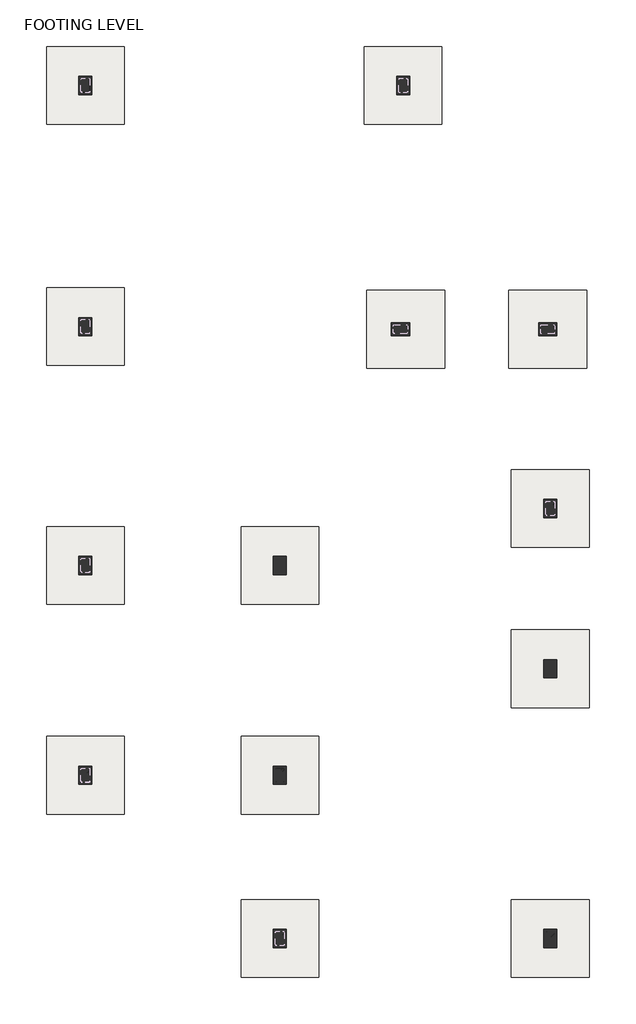
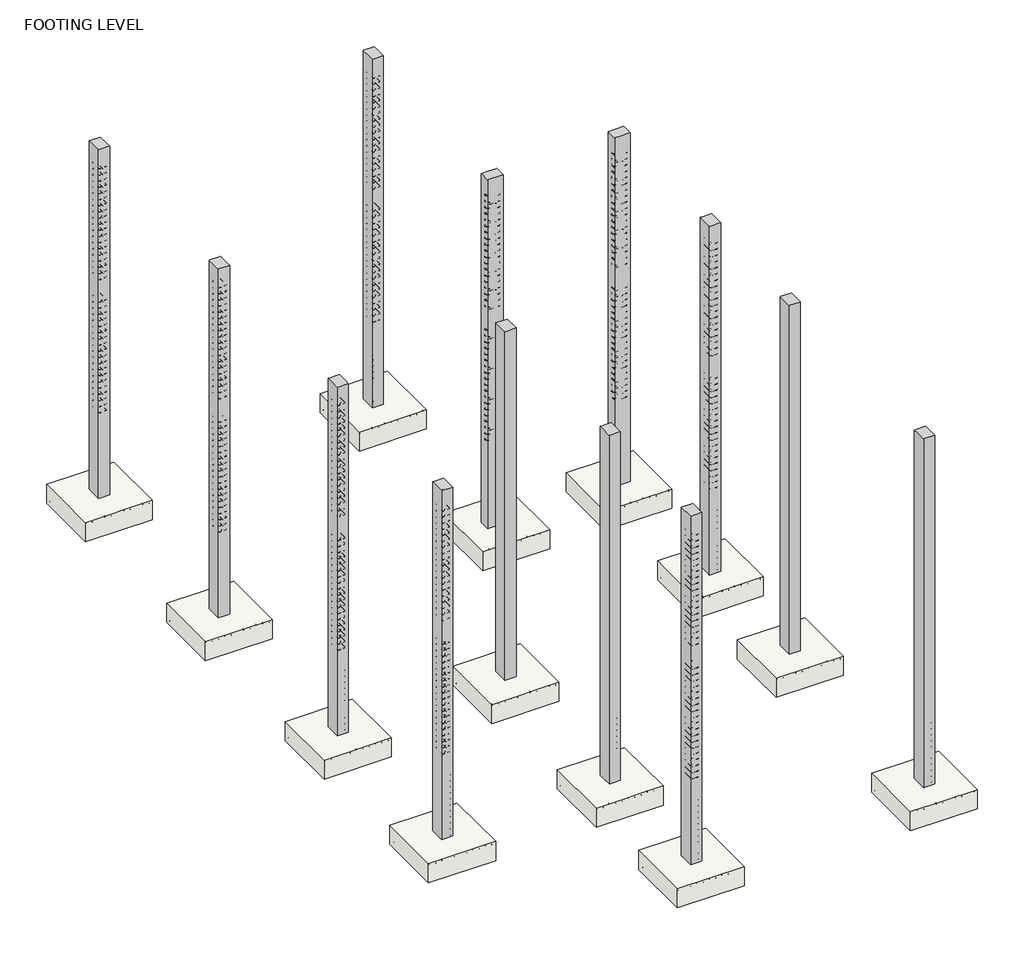
# One storey, part 1 of 9: 13 columns, 13 slabs.
"""IFC4 building model written with IfcOpenShell, lengths in millimetres."""

from ifc_helpers import new_model, si_unit, origin, place, context, project, spatial, faceted_brep, transform, mapped, element, save
from components import footing_rectangular_5_x_5_df1ede25

model = new_model("IFC4")

# Units and contexts
model_context = context("Model", 3, world=origin())
ifc_project = project(units=[si_unit("LENGTHUNIT", "METRE", prefix="MILLI")], contexts=[model_context])

# Site, building, storey
site = spatial("IfcSite", under=ifc_project)
building = spatial("IfcBuilding", under=site)
storey = spatial("IfcBuildingStorey", under=building, Name="FOOTING LEVEL", Elevation=-1981.2)

# Columns
placement = place(None, origin())
element("IfcColumn", 1, ObjectType="Concrete-Rectangular-Column : 10\" x 14\"", at=placement, inside=storey, context=model_context, shape_type="Brep", body=[
    faceted_brep([(-12235.0833659, -383.2216598, -1981.2), (-12235.0833659, -738.8216598, -1981.2), (-12489.0833659, -738.8216598, -1981.2), (-12489.0833659, -383.2216598, -1981.2), (-12235.0833659, -383.2216598, 6400.8), (-12235.0833659, -497.5216598, 6400.8), (-12235.0833659, -726.1216598, 6400.8), (-12235.0833659, -738.8216598, 6400.8), (-12489.0833659, -738.8216598, 6400.8), (-12489.0833659, -383.2216598, 6400.8), (-12476.3833659, -383.2216598, 6400.8), (-12247.7833659, -383.2216598, 6400.8)], [[[0, 1, 2, 3]], [[4, 5, 6, 7, 1, 0]], [[7, 8, 2, 1]], [[8, 9, 3, 2]], [[9, 10, 11, 4, 0, 3]], [[4, 11, 10, 9, 8, 7, 6, 5]]]),
])
element("IfcColumn", 2, ObjectType="Concrete-Rectangular-Column : 10\" x 14\"", at=placement, inside=storey, context=model_context, shape_type="Brep", body=[
    faceted_brep([(-12235.0833659, 3725.2283402, -1981.2), (-12235.0833659, 3369.6283402, -1981.2), (-12489.0833659, 3369.6283402, -1981.2), (-12489.0833659, 3725.2283402, -1981.2), (-12235.0833659, 3725.2283402, 6400.8), (-12235.0833659, 3712.5283402, 6400.8), (-12235.0833659, 3483.9283402, 6400.8), (-12235.0833659, 3369.6283402, 6400.8), (-12247.7833659, 3369.6283402, 6400.8), (-12476.3833659, 3369.6283402, 6400.8), (-12489.0833659, 3369.6283402, 6400.8), (-12489.0833659, 3725.2283402, 6400.8), (-12476.3833659, 3725.2283402, 6400.8), (-12247.7833659, 3725.2283402, 6400.8)], [[[0, 1, 2, 3]], [[4, 5, 6, 7, 1, 0]], [[7, 8, 9, 10, 2, 1]], [[10, 11, 3, 2]], [[11, 12, 13, 4, 0, 3]], [[4, 13, 12, 11, 10, 9, 8, 7, 6, 5]]]),
])
element("IfcColumn", 3, ObjectType="Concrete-Rectangular-Column : 10\" x 14\"", at=placement, inside=storey, context=model_context, shape_type="Brep", body=[
    faceted_brep([(-8425.0833659, 3725.2283402, -1981.2), (-8425.0833659, 3369.6283402, -1981.2), (-8679.0833659, 3369.6283402, -1981.2), (-8679.0833659, 3725.2283402, -1981.2), (-8425.0833659, 3725.2283402, 6400.8), (-8425.0833659, 3369.6283402, 6400.8), (-8437.7833659, 3369.6283402, 6400.8), (-8666.3833659, 3369.6283402, 6400.8), (-8679.0833659, 3369.6283402, 6400.8), (-8679.0833659, 3483.9283402, 6400.8), (-8679.0833659, 3712.5283402, 6400.8), (-8679.0833659, 3725.2283402, 6400.8)], [[[0, 1, 2, 3]], [[4, 5, 1, 0]], [[5, 6, 7, 8, 2, 1]], [[8, 9, 10, 11, 3, 2]], [[11, 4, 0, 3]], [[4, 11, 10, 9, 8, 7, 6, 5]]]),
])
element("IfcColumn", 4, ObjectType="Concrete-Rectangular-Column : 10\" x 14\"", at=placement, inside=storey, context=model_context, shape_type="Brep", body=[
    faceted_brep([(-3129.3191189, 1700.3598175, -1981.2), (-3129.3191189, 1344.7598175, -1981.2), (-3383.3191189, 1344.7598175, -1981.2), (-3383.3191189, 1700.3598175, -1981.2), (-3129.3191189, 1700.3598175, 6400.8), (-3129.3191189, 1344.7598175, 6400.8), (-3142.0191189, 1344.7598175, 6400.8), (-3370.6191189, 1344.7598175, 6400.8), (-3383.3191189, 1344.7598175, 6400.8), (-3383.3191189, 1700.3598175, 6400.8), (-3370.6191189, 1700.3598175, 6400.8), (-3142.0191189, 1700.3598175, 6400.8)], [[[0, 1, 2, 3]], [[4, 5, 1, 0]], [[5, 6, 7, 8, 2, 1]], [[8, 9, 3, 2]], [[9, 10, 11, 4, 0, 3]], [[4, 11, 10, 9, 8, 7, 6, 5]]]),
])
element("IfcColumn", 5, ObjectType="Concrete-Rectangular-Column : 10\" x 14\"", at=placement, inside=storey, context=model_context, shape_type="Brep", body=[
    faceted_brep([(-3129.3191189, -3583.6216598, -1981.2), (-3129.3191189, -3939.2216598, -1981.2), (-3383.3191189, -3939.2216598, -1981.2), (-3383.3191189, -3583.6216598, -1981.2), (-3129.3191189, -3583.6216598, 6400.8), (-3129.3191189, -3939.2216598, 6400.8), (-3383.3191189, -3939.2216598, 6400.8), (-3383.3191189, -3926.5216598, 6400.8), (-3383.3191189, -3697.9216598, 6400.8), (-3383.3191189, -3583.6216598, 6400.8), (-3370.6191189, -3583.6216598, 6400.8), (-3142.0191189, -3583.6216598, 6400.8)], [[[0, 1, 2, 3]], [[4, 5, 1, 0]], [[5, 6, 2, 1]], [[6, 7, 8, 9, 3, 2]], [[9, 10, 11, 4, 0, 3]], [[4, 11, 10, 9, 8, 7, 6, 5]]]),
])
element("IfcColumn", 6, ObjectType="Concrete-Rectangular-Column : 10\" x 14\"", at=placement, inside=storey, context=model_context, shape_type="Brep", body=[
    faceted_brep([(-8425.0833659, -3583.6216598, -1981.2), (-8425.0833659, -3939.2216598, -1981.2), (-8679.0833659, -3939.2216598, -1981.2), (-8679.0833659, -3583.6216598, -1981.2), (-8425.0833659, -3583.6216598, 6400.8), (-8425.0833659, -3697.9216598, 6400.8), (-8425.0833659, -3926.5216598, 6400.8), (-8425.0833659, -3939.2216598, 6400.8), (-8679.0833659, -3939.2216598, 6400.8), (-8679.0833659, -3583.6216598, 6400.8), (-8666.3833659, -3583.6216598, 6400.8), (-8437.7833659, -3583.6216598, 6400.8)], [[[0, 1, 2, 3]], [[4, 5, 6, 7, 1, 0]], [[7, 8, 2, 1]], [[8, 9, 3, 2]], [[9, 10, 11, 4, 0, 3]], [[4, 11, 10, 9, 8, 7, 6, 5]]]),
])
element("IfcColumn", 7, ObjectType="Concrete-Rectangular-Column : 10\" x 14\"", at=placement, inside=storey, context=model_context, shape_type="Brep", body=[
    faceted_brep([(-3129.3191189, 4841.8494441, -1981.2), (-3129.3191189, 4486.2494441, -1981.2), (-3383.3191189, 4486.2494441, -1981.2), (-3383.3191189, 4841.8494441, -1981.2), (-3129.3191189, 4841.8494441, 6400.8), (-3129.3191189, 4486.2494441, 6400.8), (-3142.0191189, 4486.2494441, 6400.8), (-3370.6191189, 4486.2494441, 6400.8), (-3383.3191189, 4486.2494441, 6400.8), (-3383.3191189, 4841.8494441, 6400.8), (-3370.6191189, 4841.8494441, 6400.8), (-3142.0191189, 4841.8494441, 6400.8)], [[[0, 1, 2, 3]], [[4, 5, 1, 0]], [[5, 6, 7, 8, 2, 1]], [[8, 9, 3, 2]], [[9, 10, 11, 4, 0, 3]], [[4, 11, 10, 9, 8, 7, 6, 5]]]),
])
element("IfcColumn", 8, ObjectType="Concrete-Rectangular-Column : 10\" x 14\"", at=placement, inside=storey, context=model_context, shape_type="Brep", body=[
    faceted_brep([(-3484.7833659, 8303.5783402, -1981.2), (-3129.1833659, 8303.5783402, -1981.2), (-3129.1833659, 8049.5783402, -1981.2), (-3484.7833659, 8049.5783402, -1981.2), (-3484.7833659, 8303.5783402, 6400.8), (-3129.1833659, 8303.5783402, 6400.8), (-3129.1833659, 8049.5783402, 6400.8), (-3142.0191189, 8049.5783402, 6400.8), (-3370.6191189, 8049.5783402, 6400.8), (-3484.7833659, 8049.5783402, 6400.8), (-3484.7833659, 8062.2783402, 6400.8), (-3484.7833659, 8290.8783402, 6400.8)], [[[0, 1, 2, 3]], [[4, 5, 1, 0]], [[5, 6, 2, 1]], [[6, 7, 8, 9, 3, 2]], [[9, 10, 11, 4, 0, 3]], [[4, 11, 10, 9, 8, 7, 6, 5]]]),
])
element("IfcColumn", 9, ObjectType="Concrete-Rectangular-Column : 10\" x 14\"", at=placement, inside=storey, context=model_context, shape_type="Brep", body=[
    faceted_brep([(-6367.6833659, 8303.5783402, -1981.2), (-6012.0833659, 8303.5783402, -1981.2), (-6012.0833659, 8049.5783402, -1981.2), (-6367.6833659, 8049.5783402, -1981.2), (-6367.6833659, 8303.5783402, 6400.8), (-6253.3833659, 8303.5783402, 6400.8), (-6024.7833659, 8303.5783402, 6400.8), (-6012.0833659, 8303.5783402, 6400.8), (-6012.0833659, 8290.8783402, 6400.8), (-6012.0833659, 8062.2783402, 6400.8), (-6012.0833659, 8049.5783402, 6400.8), (-6367.6833659, 8049.5783402, 6400.8), (-6367.6833659, 8062.2783402, 6400.8), (-6367.6833659, 8290.8783402, 6400.8)], [[[0, 1, 2, 3]], [[4, 5, 6, 7, 1, 0]], [[7, 8, 9, 10, 2, 1]], [[10, 11, 3, 2]], [[11, 12, 13, 4, 0, 3]], [[4, 13, 12, 11, 10, 9, 8, 7, 6, 5]]]),
])
element("IfcColumn", 10, ObjectType="Concrete-Rectangular-Column : 10\" x 14\"", at=placement, inside=storey, context=model_context, shape_type="Brep", body=[
    faceted_brep([(-12489.0833659, 8049.5783402, -1981.2), (-12489.0833659, 8405.1783402, -1981.2), (-12235.0833659, 8405.1783402, -1981.2), (-12235.0833659, 8049.5783402, -1981.2), (-12489.0833659, 8049.5783402, 6400.8), (-12489.0833659, 8405.1783402, 6400.8), (-12476.3833659, 8405.1783402, 6400.8), (-12247.7833659, 8405.1783402, 6400.8), (-12235.0833659, 8405.1783402, 6400.8), (-12235.0833659, 8290.8783402, 6400.8), (-12235.0833659, 8062.2783402, 6400.8), (-12235.0833659, 8049.5783402, 6400.8), (-12247.7833659, 8049.5783402, 6400.8), (-12476.3833659, 8049.5783402, 6400.8)], [[[0, 1, 2, 3]], [[4, 5, 1, 0]], [[5, 6, 7, 8, 2, 1]], [[8, 9, 10, 11, 3, 2]], [[11, 12, 13, 4, 0, 3]], [[4, 13, 12, 11, 10, 9, 8, 7, 6, 5]]]),
])
element("IfcColumn", 11, ObjectType="Concrete-Rectangular-Column : 10\" x 14\"", at=placement, inside=storey, context=model_context, shape_type="Brep", body=[
    faceted_brep([(-12489.0833659, 12773.9783402, -1981.2), (-12489.0833659, 13129.5783402, -1981.2), (-12235.0833659, 13129.5783402, -1981.2), (-12235.0833659, 12773.9783402, -1981.2), (-12489.0833659, 12773.9783402, 6400.8), (-12489.0833659, 13129.5783402, 6400.8), (-12235.0833659, 13129.5783402, 6400.8), (-12235.0833659, 13116.8783402, 6400.8), (-12235.0833659, 12888.2783402, 6400.8), (-12235.0833659, 12773.9783402, 6400.8), (-12247.7833659, 12773.9783402, 6400.8), (-12476.3833659, 12773.9783402, 6400.8)], [[[0, 1, 2, 3]], [[4, 5, 1, 0]], [[5, 6, 2, 1]], [[6, 7, 8, 9, 3, 2]], [[9, 10, 11, 4, 0, 3]], [[4, 11, 10, 9, 8, 7, 6, 5]]]),
])
element("IfcColumn", 12, ObjectType="Concrete-Rectangular-Column : 10\" x 14\"", at=placement, inside=storey, context=model_context, shape_type="Brep", body=[
    faceted_brep([(-6266.0833659, 12773.9783402, -1981.2), (-6266.0833659, 13129.5783402, -1981.2), (-6012.0833659, 13129.5783402, -1981.2), (-6012.0833659, 12773.9783402, -1981.2), (-6266.0833659, 12773.9783402, 6400.8), (-6266.0833659, 12888.2783402, 6400.8), (-6266.0833659, 13116.8783402, 6400.8), (-6266.0833659, 13129.5783402, 6400.8), (-6012.0833659, 13129.5783402, 6400.8), (-6012.0833659, 12773.9783402, 6400.8), (-6024.7833659, 12773.9783402, 6400.8), (-6253.3833659, 12773.9783402, 6400.8)], [[[0, 1, 2, 3]], [[4, 5, 6, 7, 1, 0]], [[7, 8, 2, 1]], [[8, 9, 3, 2]], [[9, 10, 11, 4, 0, 3]], [[4, 11, 10, 9, 8, 7, 6, 5]]]),
])
element("IfcColumn", 13, ObjectType="Concrete-Rectangular-Column : 10\" x 14\"", at=placement, inside=storey, context=model_context, shape_type="Brep", body=[
    faceted_brep([(-8425.0833659, -383.2216598, -1981.2), (-8425.0833659, -738.8216598, -1981.2), (-8679.0833659, -738.8216598, -1981.2), (-8679.0833659, -383.2216598, -1981.2), (-8425.0833659, -383.2216598, 6400.8), (-8425.0833659, -738.8216598, 6400.8), (-8437.7833659, -738.8216598, 6400.8), (-8666.3833659, -738.8216598, 6400.8), (-8679.0833659, -738.8216598, 6400.8), (-8679.0833659, -726.1216598, 6400.8), (-8679.0833659, -497.5216598, 6400.8), (-8679.0833659, -383.2216598, 6400.8), (-8666.3833659, -383.2216598, 6400.8), (-8437.7833659, -383.2216598, 6400.8)], [[[0, 1, 2, 3]], [[4, 5, 1, 0]], [[5, 6, 7, 8, 2, 1]], [[8, 9, 10, 11, 3, 2]], [[11, 12, 13, 4, 0, 3]], [[4, 13, 12, 11, 10, 9, 8, 7, 6, 5]]]),
])

# Slabs
footing_rectangular_5_x_5_shape = footing_rectangular_5_x_5_df1ede25(model_context)
element("IfcSlab", 14, ObjectType="Footing-Rectangular : 5' x 5'", at=placement, inside=storey, context=model_context, shape_type="MappedRepresentation", body=[
    mapped(footing_rectangular_5_x_5_shape, transform((-12362.0833659, -561.0216598, -1981.2), x_axis=(1.0, 0.0, 0.0), y_axis=(0.0, 1.0, 0.0), z_axis=(0.0, 0.0, 1.0))),
])
element("IfcSlab", 15, ObjectType="Footing-Rectangular : 5' x 5'", at=placement, inside=storey, context=model_context, shape_type="MappedRepresentation", body=[
    mapped(footing_rectangular_5_x_5_shape, transform((-12362.0833659, 3547.4283402, -1981.2), x_axis=(1.0, 0.0, 0.0), y_axis=(0.0, 1.0, 0.0), z_axis=(0.0, 0.0, 1.0))),
])
element("IfcSlab", 16, ObjectType="Footing-Rectangular : 5' x 5'", at=placement, inside=storey, context=model_context, shape_type="MappedRepresentation", body=[
    mapped(footing_rectangular_5_x_5_shape, transform((-8552.0833659, 3547.4283402, -1981.2), x_axis=(1.0, 0.0, 0.0), y_axis=(0.0, 1.0, 0.0), z_axis=(0.0, 0.0, 1.0))),
])
element("IfcSlab", 17, ObjectType="Footing-Rectangular : 5' x 5'", at=placement, inside=storey, context=model_context, shape_type="MappedRepresentation", body=[
    mapped(footing_rectangular_5_x_5_shape, transform((-8552.0833659, -561.0216598, -1981.2), x_axis=(1.0, 0.0, 0.0), y_axis=(0.0, 1.0, 0.0), z_axis=(0.0, 0.0, 1.0))),
])
element("IfcSlab", 18, ObjectType="Footing-Rectangular : 5' x 5'", at=placement, inside=storey, context=model_context, shape_type="MappedRepresentation", body=[
    mapped(footing_rectangular_5_x_5_shape, transform((-8552.0833659, -3761.4216598, -1981.2), x_axis=(1.0, 0.0, 0.0), y_axis=(0.0, 1.0, 0.0), z_axis=(0.0, 0.0, 1.0))),
])
element("IfcSlab", 19, ObjectType="Footing-Rectangular : 5' x 5'", at=placement, inside=storey, context=model_context, shape_type="MappedRepresentation", body=[
    mapped(footing_rectangular_5_x_5_shape, transform((-3256.3191189, -3761.4216598, -1981.2), x_axis=(1.0, 0.0, 0.0), y_axis=(0.0, 1.0, 0.0), z_axis=(0.0, 0.0, 1.0))),
])
element("IfcSlab", 20, ObjectType="Footing-Rectangular : 5' x 5'", at=placement, inside=storey, context=model_context, shape_type="MappedRepresentation", body=[
    mapped(footing_rectangular_5_x_5_shape, transform((-3256.3191189, 1522.5598175, -1981.2), x_axis=(1.0, 0.0, 0.0), y_axis=(0.0, 1.0, 0.0), z_axis=(0.0, 0.0, 1.0))),
])
element("IfcSlab", 21, ObjectType="Footing-Rectangular : 5' x 5'", at=placement, inside=storey, context=model_context, shape_type="MappedRepresentation", body=[
    mapped(footing_rectangular_5_x_5_shape, transform((-3256.3191189, 4664.0494441, -1981.2), x_axis=(1.0, 0.0, 0.0), y_axis=(0.0, 1.0, 0.0), z_axis=(0.0, 0.0, 1.0))),
])
element("IfcSlab", 22, ObjectType="Footing-Rectangular : 5' x 5'", at=placement, inside=storey, context=model_context, shape_type="MappedRepresentation", body=[
    mapped(footing_rectangular_5_x_5_shape, transform((-6088.2833659, 8176.5783402, -1981.2), x_axis=(1.0, 0.0, 0.0), y_axis=(0.0, 1.0, 0.0), z_axis=(0.0, 0.0, 1.0))),
])
element("IfcSlab", 23, ObjectType="Footing-Rectangular : 5' x 5'", at=placement, inside=storey, context=model_context, shape_type="MappedRepresentation", body=[
    mapped(footing_rectangular_5_x_5_shape, transform((-3306.9833659, 8176.5783402, -1981.2), x_axis=(1.0, 0.0, 0.0), y_axis=(0.0, 1.0, 0.0), z_axis=(0.0, 0.0, 1.0))),
])
element("IfcSlab", 24, ObjectType="Footing-Rectangular : 5' x 5'", at=placement, inside=storey, context=model_context, shape_type="MappedRepresentation", body=[
    mapped(footing_rectangular_5_x_5_shape, transform((-12362.0833659, 8227.3783402, -1981.2), x_axis=(1.0, 0.0, 0.0), y_axis=(0.0, 1.0, 0.0), z_axis=(0.0, 0.0, 1.0))),
])
element("IfcSlab", 25, ObjectType="Footing-Rectangular : 5' x 5'", at=placement, inside=storey, context=model_context, shape_type="MappedRepresentation", body=[
    mapped(footing_rectangular_5_x_5_shape, transform((-12362.0833659, 12951.7783402, -1981.2), x_axis=(1.0, 0.0, 0.0), y_axis=(0.0, 1.0, 0.0), z_axis=(0.0, 0.0, 1.0))),
])
element("IfcSlab", 26, ObjectType="Footing-Rectangular : 5' x 5'", at=placement, inside=storey, context=model_context, shape_type="MappedRepresentation", body=[
    mapped(footing_rectangular_5_x_5_shape, transform((-6139.0833659, 12951.7783402, -1981.2), x_axis=(1.0, 0.0, 0.0), y_axis=(0.0, 1.0, 0.0), z_axis=(0.0, 0.0, 1.0))),
])

save(model, "model.ifc")

# Revit data of these elements
# Grids (mm)
#   "1": line (-12362.083, -8662.366) -> (-12362.083, 19256.895)
#   "3": line (-8552.083, -8662.366) -> (-8552.083, 19256.895)
#   "4": line (-6139.083, -8662.366) -> (-6139.083, 19256.895)
#   "6": line (-3256.319, -8662.366) -> (-3256.319, 19256.895)
#   "7": line (4582.098, 3547.428) -> (-17928.309, 3547.428)
#   "2": line (4582.098, -561.022) -> (-17928.309, -561.022)
#   "8": line (4582.098, 8227.378) -> (-17928.309, 8227.378)
#   "9": line (4582.098, 4664.049) -> (-17928.309, 4664.049)
#   "10": line (4582.098, 12951.778) -> (-17928.309, 12951.778)
# Type "Concrete-Rectangular-Column : 10\" x 14\""
#   Assembly Code = "B10"
#   b = 0' - 10"
#   h = 1' - 2"
#   Structural Material [instance default] = Concrete, Cast-in-Place gray
# Type "Footing-Rectangular : 5' x 5'"
#   Assembly Code = "A1010100"
#   Width = 5' - 0"
#   Length = 5' - 0"
#   Foundation Thickness = 1' - 6"
#   Structural Material [instance default] = Concrete, Cast-in-Place gray
# Elements 1, 2, 3, 4, 5, 6, 7, 8, 9, 10, 11, 12, 13 (IfcColumn, "Concrete-Rectangular-Column : 10\" x 14\"")
#   Structural Material = Concrete, Cast-in-Place gray
#   Phase Created = New Construction
#   Materials on its faces: "Concrete, Cast-in-Place gray"
# Elements 14, 15, 16, 17, 18, 19, 20, 21, 22, 23, 24, 25, 26 (IfcSlab, "Footing-Rectangular : 5' x 5'")
#   Structural Material = Concrete, Cast-in-Place gray
#   Phase Created = New Construction
#   Materials on its faces: "Concrete, Cast-in-Place gray"
# Materials
#   "Concrete, Cast-in-Place gray": class "Concrete", colour RGB 192 192 192, transparency 0, Description = "Cast-in-place concrete", Cost = 0
